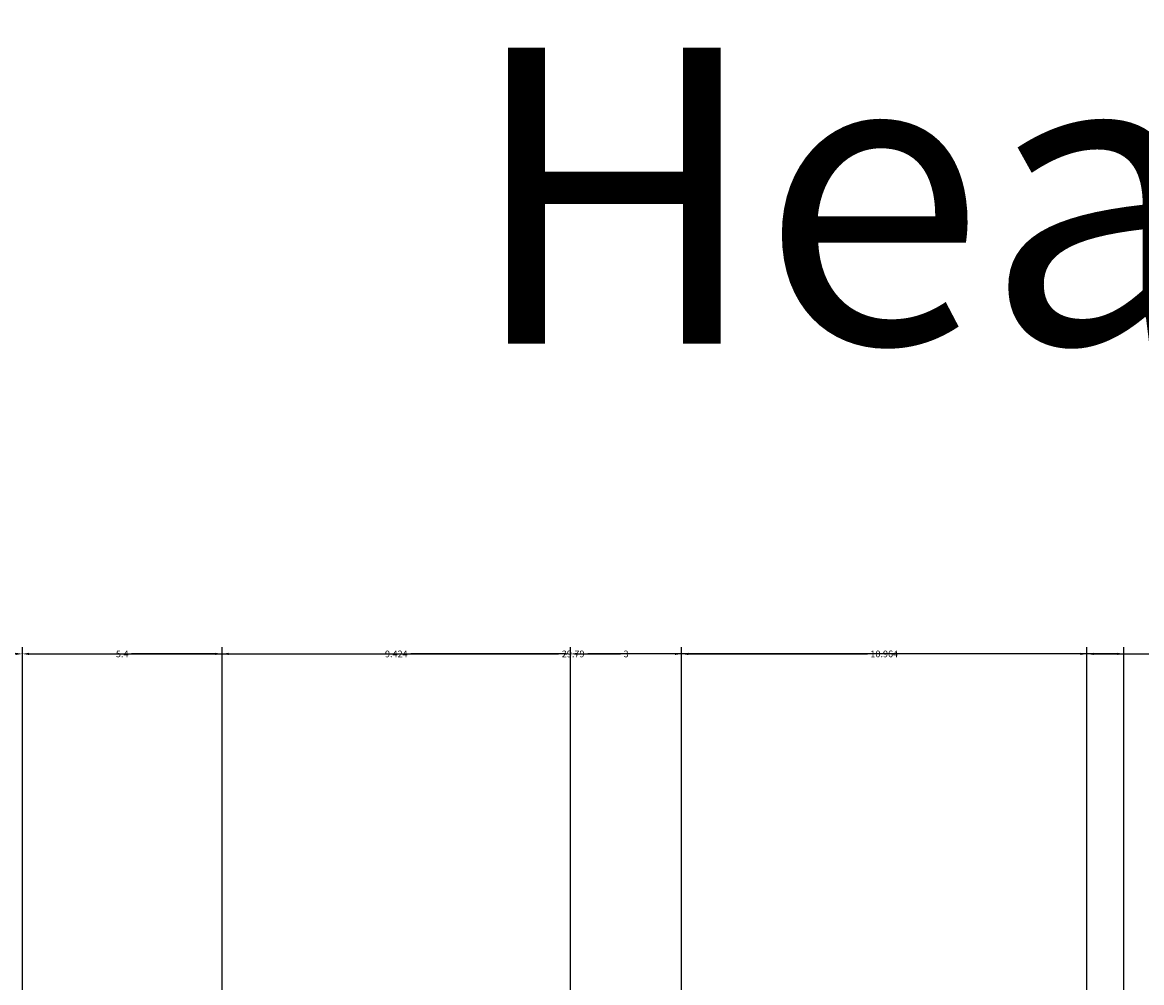
# Model space of a CAD drawing. Units: inches. Extents: x -12 to 334, y -10 to 186.
# Tile 27 of 77: x 58 to 88, y 160 to 186. Entities that reach past the tile are written whole.
import ezdxf

# ---------------------------------------------------------------- set-up
doc = ezdxf.new("R2010")
doc.units = ezdxf.units.IN
doc.header["$MEASUREMENT"] = 0
doc.layers.add('M-ANNO-TEXT', color=3, linetype='Continuous', lineweight=25)
doc.layers.add('M-DIMS', color=2, linetype='Continuous', lineweight=18)
doc.styles.get("Standard").update_dxf_attribs({"font": 'arial.ttf'})
doc.dimstyles.get("Standard").update_dxf_attribs({"dimtxt": 0.18, "dimasz": 0.18, "dimexe": 0.18, "dimexo": 0.0625, "dimgap": 0.09, "dimtad": 0, "dimtih": 1, "dimtoh": 1, "dimdec": 4, "dimzin": 0, "dimdsep": 46, "dimtxsty": 'Standard', "dimcen": 0.09, "dimadec": 0, "dimazin": 0, "dimtfac": 1, "dimtdec": 4, "dimtofl": 0, "dimtmove": 0, "dimatfit": 3, "dimfxl": 1, "dimtolj": 1, "dimtzin": 0, "dimarcsym": 0})

# ---------------------------------------------------------------- blocks, each defined once
blk = doc.blocks.new('*D3')
at = {"layer": 'Defpoints', "color": 0, "transparency": 16777216}
for p in [(58.1, 169.385), (32.1, 127.708), (58.1, 127.708)]:
    blk.add_point(p, dxfattribs=at)
at = {"layer": 'M-DIMS', "color": 0, "lineweight": -2, "transparency": 16777216}
for p, q in [((32.1, 127.77), (32.1, 169.565)), ((58.1, 127.77), (58.1, 169.565)), ((32.28, 169.385), (44.88, 169.385)), ((57.92, 169.385), (45.321, 169.385))]:
    blk.add_line(p, q, dxfattribs=at)
at = {"layer": 'M-DIMS', "color": 0, "transparency": 16777216}
for points in [[(32.28, 169.415), (32.28, 169.355), (32.1, 169.385)], [(57.92, 169.415), (57.92, 169.355), (58.1, 169.385)]]:
    blk.add_solid(points, dxfattribs=at)
at = {"layer": 'M-DIMS', "color": 0, "transparency": 16777216, "insert": (45.1, 169.385), "char_height": 0.18, "attachment_point": 5}
blk.add_mtext('\\A1;26', dxfattribs=at)
blk = doc.blocks.new('*D10')
at = {"layer": 'Defpoints', "color": 0, "transparency": 16777216}
for p in [(63.5, 169.385), (58.1, 127.708), (63.5, 109.058)]:
    blk.add_point(p, dxfattribs=at)
at = {"layer": 'M-DIMS', "color": 0, "lineweight": -2, "transparency": 16777216}
for p, q in [((58.1, 127.77), (58.1, 169.565)), ((63.5, 109.121), (63.5, 169.565)), ((58.28, 169.385), (60.547, 169.385)), ((63.32, 169.385), (61.054, 169.385))]:
    blk.add_line(p, q, dxfattribs=at)
at = {"layer": 'M-DIMS', "color": 0, "transparency": 16777216}
for points in [[(58.28, 169.415), (58.28, 169.355), (58.1, 169.385)], [(63.32, 169.415), (63.32, 169.355), (63.5, 169.385)]]:
    blk.add_solid(points, dxfattribs=at)
at = {"layer": 'M-DIMS', "color": 0, "transparency": 16777216, "insert": (60.8, 169.385), "char_height": 0.18, "attachment_point": 5}
blk.add_mtext('\\A1;5.4', dxfattribs=at)
blk = doc.blocks.new('*D11')
at = {"layer": 'Defpoints', "color": 0, "transparency": 16777216}
for p in [(72.924, 169.385), (63.5, 109.058), (72.924, 109.058)]:
    blk.add_point(p, dxfattribs=at)
at = {"layer": 'M-DIMS', "color": 0, "lineweight": -2, "transparency": 16777216}
for p, q in [((63.5, 109.121), (63.5, 169.565)), ((72.924, 109.121), (72.924, 169.565)), ((63.68, 169.385), (67.819, 169.385)), ((72.744, 169.385), (68.606, 169.385))]:
    blk.add_line(p, q, dxfattribs=at)
at = {"layer": 'M-DIMS', "color": 0, "transparency": 16777216}
for points in [[(63.68, 169.415), (63.68, 169.355), (63.5, 169.385)], [(72.744, 169.415), (72.744, 169.355), (72.924, 169.385)]]:
    blk.add_solid(points, dxfattribs=at)
at = {"layer": 'M-DIMS', "color": 0, "transparency": 16777216, "insert": (68.212, 169.385), "char_height": 0.18, "attachment_point": 5}
blk.add_mtext('\\A1;9.424', dxfattribs=at)
blk = doc.blocks.new('*D12')
at = {"layer": 'Defpoints', "color": 0, "transparency": 16777216}
for p in [(75.924, 169.385), (72.924, 109.058), (75.924, 109.058)]:
    blk.add_point(p, dxfattribs=at)
at = {"layer": 'M-DIMS', "color": 0, "lineweight": -2, "transparency": 16777216}
for p, q in [((72.924, 109.121), (72.924, 169.565)), ((75.924, 109.121), (75.924, 169.565)), ((73.104, 169.385), (74.275, 169.385)), ((75.744, 169.385), (74.573, 169.385))]:
    blk.add_line(p, q, dxfattribs=at)
at = {"layer": 'M-DIMS', "color": 0, "transparency": 16777216}
for points in [[(73.104, 169.415), (73.104, 169.355), (72.924, 169.385)], [(75.744, 169.415), (75.744, 169.355), (75.924, 169.385)]]:
    blk.add_solid(points, dxfattribs=at)
at = {"layer": 'M-DIMS', "color": 0, "transparency": 16777216, "insert": (74.424, 169.385), "char_height": 0.18, "attachment_point": 5}
blk.add_mtext('\\A1;3', dxfattribs=at)
blk = doc.blocks.new('*D13')
at = {"layer": 'Defpoints', "color": 0, "transparency": 16777216}
for p in [(86.888, 169.385), (75.924, 109.058), (86.888, 109.058)]:
    blk.add_point(p, dxfattribs=at)
at = {"layer": 'M-DIMS', "color": 0, "lineweight": -2, "transparency": 16777216}
for p, q in [((75.924, 109.121), (75.924, 169.565)), ((86.888, 109.121), (86.888, 169.565)), ((76.104, 169.385), (80.951, 169.385)), ((86.708, 169.385), (81.861, 169.385))]:
    blk.add_line(p, q, dxfattribs=at)
at = {"layer": 'M-DIMS', "color": 0, "transparency": 16777216}
for points in [[(76.104, 169.415), (76.104, 169.355), (75.924, 169.385)], [(86.708, 169.415), (86.708, 169.355), (86.888, 169.385)]]:
    blk.add_solid(points, dxfattribs=at)
at = {"layer": 'M-DIMS', "color": 0, "transparency": 16777216, "insert": (81.406, 169.385), "char_height": 0.18, "attachment_point": 5}
blk.add_mtext('\\A1;10.964', dxfattribs=at)
blk = doc.blocks.new('*D15')
at = {"layer": 'Defpoints', "color": 0, "transparency": 16777216}
for p in [(106.177, 169.385), (86.888, 109.058), (106.177, 102.896)]:
    blk.add_point(p, dxfattribs=at)
at = {"layer": 'M-DIMS', "color": 0, "lineweight": -2, "transparency": 16777216}
for p, q in [((86.888, 109.121), (86.888, 169.565)), ((106.177, 102.958), (106.177, 169.565)), ((87.068, 169.385), (96.147, 169.385)), ((105.997, 169.385), (96.918, 169.385))]:
    blk.add_line(p, q, dxfattribs=at)
at = {"layer": 'M-DIMS', "color": 0, "transparency": 16777216}
for points in [[(87.068, 169.415), (87.068, 169.355), (86.888, 169.385)], [(105.997, 169.415), (105.997, 169.355), (106.177, 169.385)]]:
    blk.add_solid(points, dxfattribs=at)
at = {"layer": 'M-DIMS', "color": 0, "transparency": 16777216, "insert": (96.532, 169.385), "char_height": 0.18, "attachment_point": 5}
blk.add_mtext('\\A1;19.29', dxfattribs=at)
blk = doc.blocks.new('*D26')
at = {"layer": 'Defpoints', "color": 0, "transparency": 16777216}
for p in [(87.888, 169.385), (87.888, 56.321), (58.1, 33.675)]:
    blk.add_point(p, dxfattribs=at)
at = {"layer": 'M-DIMS', "color": 0, "lineweight": -2, "transparency": 16777216}
for p, q in [((58.1, 33.738), (58.1, 169.565)), ((87.888, 56.383), (87.888, 169.565)), ((58.28, 169.385), (72.599, 169.385)), ((87.708, 169.385), (73.389, 169.385))]:
    blk.add_line(p, q, dxfattribs=at)
at = {"layer": 'M-DIMS', "color": 0, "transparency": 16777216}
for points in [[(58.28, 169.415), (58.28, 169.355), (58.1, 169.385)], [(87.708, 169.415), (87.708, 169.355), (87.888, 169.385)]]:
    blk.add_solid(points, dxfattribs=at)
at = {"layer": 'M-DIMS', "color": 0, "transparency": 16777216, "insert": (72.994, 169.385), "char_height": 0.18, "attachment_point": 5}
blk.add_mtext('\\A1;29.79', dxfattribs=at)

msp = doc.modelspace()

# ---------------------------------------------------------------- texts
at = {"layer": 'M-ANNO-TEXT', "insert": (70.1252, 185.7805), "char_height": 8, "attachment_point": 1}
msp.add_mtext_dynamic_manual_height_columns('Heat exchanger in a steam boiler', width=205.597506, gutter_width=1, heights=[0], dxfattribs=at)

# ---------------------------------------------------------------- dimensions: what is measured, and where the dimension line sits
at = {"layer": 'M-DIMS'}
for base, p1, p2, override, picture, middle in [((58.1002, 169.3845), (32.1002, 127.7078), (58.1002, 127.7078), {"dimdec": 0, "dimlfac": 1, "dimrnd": 0, "dimzin": 0, "dimdsep": 46, "dimlunit": 2}, '*D3', (45.1002, 169.3845)), ((63.5, 169.3845), (58.1002, 127.7078), (63.5, 109.0583), {"dimdec": 1, "dimlfac": 1, "dimrnd": 0, "dimzin": 0, "dimdsep": 46, "dimlunit": 2}, '*D10', (60.8001, 169.3845)), ((87.8879, 169.3845), (58.1002, 33.6752), (87.8879, 56.3205), {"dimdec": 2, "dimlfac": 1, "dimrnd": 0, "dimzin": 0, "dimdsep": 46, "dimlunit": 2}, '*D26', (72.9941, 169.3845)), ((72.9244, 169.3845), (63.5, 109.0583), (72.9244, 109.0583), {"dimdec": 3, "dimlfac": 1, "dimrnd": 0, "dimzin": 0, "dimdsep": 46, "dimlunit": 2}, '*D11', (68.2122, 169.3845)), ((75.9244, 169.3845), (72.9244, 109.0583), (75.9244, 109.0583), {"dimdec": 0, "dimlfac": 1, "dimrnd": 0, "dimzin": 0, "dimdsep": 46, "dimlunit": 2}, '*D12', (74.4244, 169.3845)), ((86.887907, 169.384532), (75.924407, 109.05834), (86.887907, 109.05834), {"dimdec": 3, "dimlfac": 1, "dimrnd": 0, "dimzin": 0, "dimdsep": 46, "dimlunit": 2}, '*D13', (81.406157, 169.384532)), ((106.1771, 169.3845), (86.8879, 109.0583), (106.1771, 102.8958), {"dimdec": 2, "dimlfac": 1, "dimrnd": 0, "dimzin": 0, "dimdsep": 46, "dimlunit": 2}, '*D15', (96.5325, 169.3845))]:
    dim = msp.add_linear_dim(base=base, p1=p1, p2=p2, dimstyle='Standard', override=override, dxfattribs=at)
    dim.commit()
    dim.dimension.update_dxf_attribs({"geometry": picture, "text_midpoint": middle})

doc.saveas('drawing.dxf')
